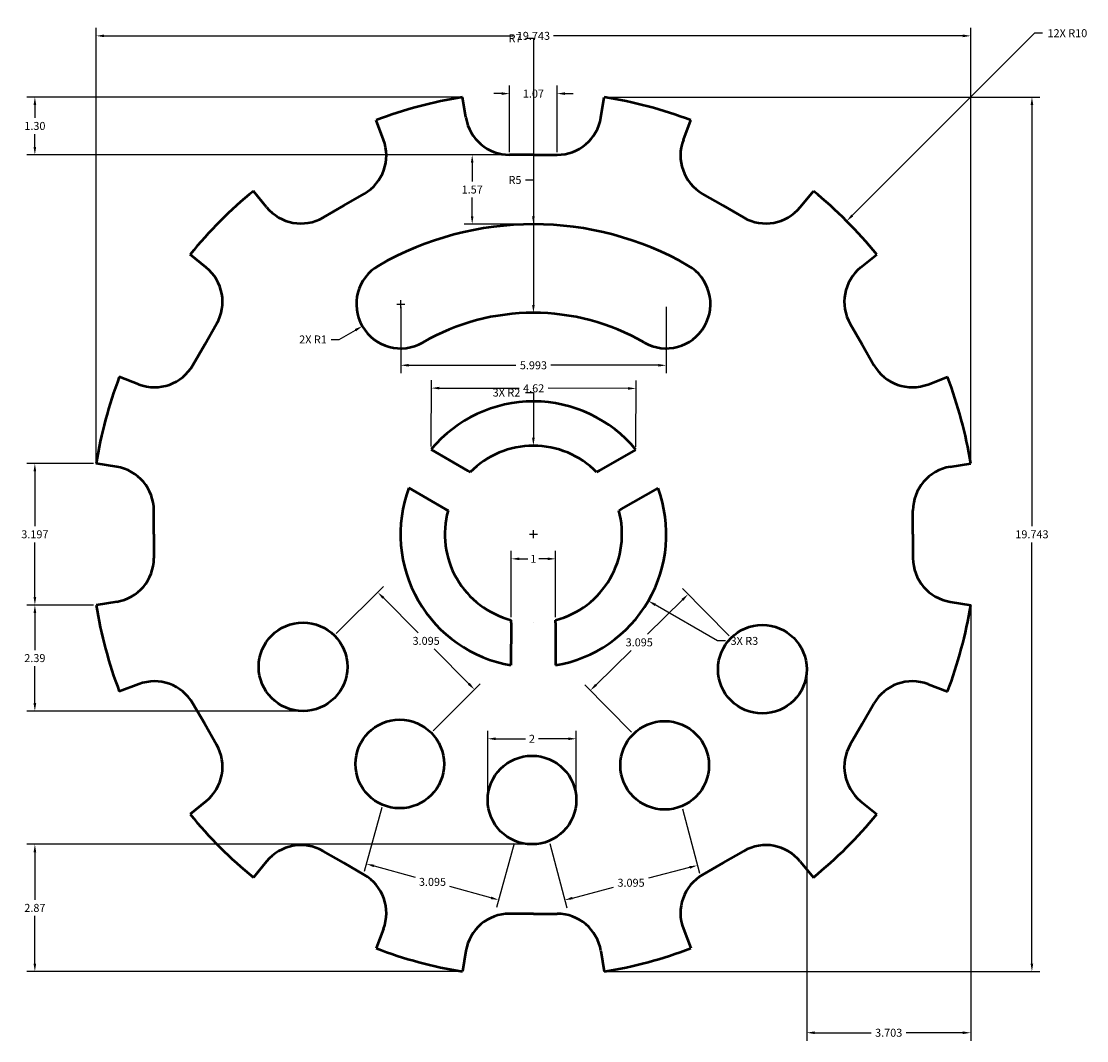
# Model space of a CAD drawing. Units: inches. Extents: x 14.9 to 39, y 2.3 to 25.3.
import ezdxf

# ---------------------------------------------------------------- set-up
doc = ezdxf.new("R2010")
doc.units = ezdxf.units.IN
doc.header["$MEASUREMENT"] = 0
for name, color, linetype, lineweight in [('M-CONS', 8, 'Continuous', 13), ('M-DIMS', 2, 'Continuous', 18), ('M-OUTL', 7, 'Continuous', 50)]:
    doc.layers.add(name, color=color, linetype=linetype, lineweight=lineweight)
doc.styles.get("Standard").update_dxf_attribs({"font": 'arial.ttf'})
doc.dimstyles.get("Standard").update_dxf_attribs({"dimtxt": 0.18, "dimasz": 0.18, "dimexe": 0.18, "dimexo": 0.0625, "dimgap": 0.09, "dimtad": 0, "dimtih": 1, "dimtoh": 1, "dimdec": 4, "dimzin": 0, "dimdsep": 46, "dimtxsty": 'Standard', "dimcen": 0.09, "dimadec": 0, "dimazin": 0, "dimtfac": 1, "dimtdec": 4, "dimtofl": 0, "dimtmove": 0, "dimatfit": 3, "dimfxl": 1, "dimtolj": 1, "dimtzin": 0, "dimarcsym": 0})

# ---------------------------------------------------------------- blocks, each defined once
blk = doc.blocks.new('*U1')
for p, q in [((-0.496, 0.479), (-0.504, -0.477)), ((0.504, 0.479), (0.501, -0.479))]:
    blk.add_line(p, q)
blk = doc.blocks.new('*U2')
at = {"layer": 'M-OUTL', "color": 0, "linetype": 'ByBlock', "lineweight": -2, "transparency": 16777216}
for p, rotation in [((24.356, 14.954), 240), ((28.65, 14.948), 120)]:
    blk.add_blockref('*U1', p, dxfattribs=dict(at, rotation=rotation))
blk.add_blockref('*U1', (26.498, 11.232), dxfattribs=at)
blk = doc.blocks.new('*U3')
blk.add_circle((0, 0), 1)
blk = doc.blocks.new('*U4')
at = {"layer": 'M-OUTL', "color": 0, "linetype": 'ByBlock', "lineweight": -2, "transparency": 16777216}
for p, rotation in [((31.67, 10.664), 119.5610080297864), ((23.484, 8.526), 29.89025200744661), ((29.464, 8.494), 89.67075602233986), ((26.469, 7.711), 59.78050401489326)]:
    blk.add_blockref('*U3', p, dxfattribs=dict(at, rotation=rotation))
blk.add_blockref('*U3', (21.301, 10.719), dxfattribs=at)
blk = doc.blocks.new('*U5')
for p, q in [((-1.523, 0.188), (-1.598, 0.652)), ((1.523, 0.188), (1.598, 0.652)), ((0, -0.652), (-0.536, -0.652)), ((0, -0.652), (0.536, -0.652))]:
    blk.add_line(p, q)
for centre, start, end in [((-0.536, 0.348), 189.1976, 270), ((0.536, 0.348), 270, 350.8024)]:
    blk.add_arc(centre, 1, start, end)
blk = doc.blocks.new('*U6')
at = {"layer": 'M-OUTL', "color": 0, "linetype": 'ByBlock', "lineweight": -2, "transparency": 16777216}
blk.add_blockref('*U5', (26.501, 22.931), dxfattribs=at)
for p, rotation in [((21.892, 21.696), 30), ((31.111, 21.696), 329.9999999999999), ((18.517, 18.321), 60), ((34.486, 18.321), 300), ((17.282, 13.711), 90), ((35.721, 13.711), 269.9999999999999), ((18.517, 9.102), 120), ((34.486, 9.102), 240), ((21.892, 5.727), 150), ((31.111, 5.727), 210), ((26.501, 4.492), 180)]:
    blk.add_blockref('*U5', p, dxfattribs=dict(at, rotation=rotation))
blk = doc.blocks.new('*D7')
at = {"layer": 'Defpoints', "color": 0, "transparency": 16777216}
for p in [(36.373, 24.965), (16.63, 15.31), (36.373, 15.31)]:
    blk.add_point(p, dxfattribs=at)
at = {"layer": 'M-DIMS', "color": 0, "lineweight": -2, "transparency": 16777216}
for p, q in [((16.63, 15.372), (16.63, 25.145)), ((36.373, 15.372), (36.373, 25.145)), ((16.81, 24.965), (26.046, 24.965)), ((36.193, 24.965), (26.957, 24.965))]:
    blk.add_line(p, q, dxfattribs=at)
at = {"layer": 'M-DIMS', "color": 0, "transparency": 16777216}
for points in [[(16.81, 24.995), (16.81, 24.935), (16.63, 24.965)], [(36.193, 24.995), (36.193, 24.935), (36.373, 24.965)]]:
    blk.add_solid(points, dxfattribs=at)
at = {"layer": 'M-DIMS', "color": 0, "transparency": 16777216, "insert": (26.501, 24.965), "char_height": 0.18, "attachment_point": 5}
blk.add_mtext('\\A1;19.743', dxfattribs=at)
blk = doc.blocks.new('*D8')
at = {"layer": 'Defpoints', "color": 0, "transparency": 16777216}
for p in [(28.1, 23.583), (37.755, 23.583), (28.1, 3.84)]:
    blk.add_point(p, dxfattribs=at)
at = {"layer": 'M-DIMS', "color": 0, "lineweight": -2, "transparency": 16777216}
for p, q in [((28.162, 23.583), (37.935, 23.583)), ((37.755, 23.403), (37.755, 13.893)), ((37.755, 4.02), (37.755, 13.529)), ((28.162, 3.84), (37.935, 3.84))]:
    blk.add_line(p, q, dxfattribs=at)
at = {"layer": 'M-DIMS', "color": 0, "transparency": 16777216}
for points in [[(37.725, 23.403), (37.785, 23.403), (37.755, 23.583)], [(37.725, 4.02), (37.785, 4.02), (37.755, 3.84)]]:
    blk.add_solid(points, dxfattribs=at)
at = {"layer": 'M-DIMS', "color": 0, "transparency": 16777216, "insert": (37.755, 13.711), "char_height": 0.18, "attachment_point": 5}
blk.add_mtext('\\A1;19.743', dxfattribs=at)
blk = doc.blocks.new('*D9')
at = {"layer": 'Defpoints', "color": 0, "transparency": 16777216}
for p in [(27.469, 9.094), (25.469, 7.711), (27.469, 7.711)]:
    blk.add_point(p, dxfattribs=at)
at = {"layer": 'M-DIMS', "color": 0, "lineweight": -2, "transparency": 16777216}
for p, q in [((25.469, 7.774), (25.469, 9.274)), ((27.469, 7.774), (27.469, 9.274)), ((25.649, 9.094), (26.32, 9.094)), ((27.289, 9.094), (26.619, 9.094))]:
    blk.add_line(p, q, dxfattribs=at)
at = {"layer": 'M-DIMS', "color": 0, "transparency": 16777216}
for points in [[(25.649, 9.124), (25.649, 9.064), (25.469, 9.094)], [(27.289, 9.124), (27.289, 9.064), (27.469, 9.094)]]:
    blk.add_solid(points, dxfattribs=at)
at = {"layer": 'M-DIMS', "color": 0, "transparency": 16777216, "insert": (26.469, 9.094), "char_height": 0.18, "attachment_point": 5}
blk.add_mtext('\\A1;2', dxfattribs=at)
blk = doc.blocks.new('*D10')
at = {"layer": 'Defpoints', "color": 0, "transparency": 16777216}
for p in [(23.505, 18.91), (29.498, 18.91), (23.505, 17.527)]:
    blk.add_point(p, dxfattribs=at)
at = {"layer": 'M-DIMS', "color": 0, "lineweight": -2, "transparency": 16777216}
for p, q in [((23.505, 18.847), (23.505, 17.347)), ((29.498, 18.847), (29.498, 17.347)), ((23.685, 17.527), (26.108, 17.527)), ((29.318, 17.527), (26.895, 17.527))]:
    blk.add_line(p, q, dxfattribs=at)
at = {"layer": 'M-DIMS', "color": 0, "transparency": 16777216}
for points in [[(23.685, 17.557), (23.685, 17.497), (23.505, 17.527)], [(29.318, 17.557), (29.318, 17.497), (29.498, 17.527)]]:
    blk.add_solid(points, dxfattribs=at)
at = {"layer": 'M-DIMS', "color": 0, "transparency": 16777216, "insert": (26.501, 17.527), "char_height": 0.18, "attachment_point": 5}
blk.add_mtext('\\A1;5.993', dxfattribs=at)
blk = doc.blocks.new('*D11')
at = {"layer": 'Defpoints', "color": 0, "transparency": 16777216}
for p in [(15.247, 15.31), (16.63, 15.31), (16.63, 12.113)]:
    blk.add_point(p, dxfattribs=at)
at = {"layer": 'M-DIMS', "color": 0, "lineweight": -2, "transparency": 16777216}
for p, q in [((16.567, 15.31), (15.067, 15.31)), ((15.247, 15.13), (15.247, 13.893)), ((15.247, 12.293), (15.247, 13.529)), ((16.567, 12.113), (15.067, 12.113))]:
    blk.add_line(p, q, dxfattribs=at)
at = {"layer": 'M-DIMS', "color": 0, "transparency": 16777216}
for points in [[(15.217, 15.13), (15.277, 15.13), (15.247, 15.31)], [(15.217, 12.293), (15.277, 12.293), (15.247, 12.113)]]:
    blk.add_solid(points, dxfattribs=at)
at = {"layer": 'M-DIMS', "color": 0, "transparency": 16777216, "insert": (15.247, 13.711), "char_height": 0.18, "attachment_point": 5}
blk.add_mtext('\\A1;3.197', dxfattribs=at)
blk = doc.blocks.new('*D12')
at = {"layer": 'Defpoints', "color": 0, "transparency": 16777216}
for p in [(24.903, 23.583), (15.247, 22.279), (25.965, 22.279)]:
    blk.add_point(p, dxfattribs=at)
at = {"layer": 'M-DIMS', "color": 0, "lineweight": -2, "transparency": 16777216}
for p, q in [((24.84, 23.583), (15.067, 23.583)), ((15.247, 23.403), (15.247, 23.113)), ((15.247, 22.459), (15.247, 22.749)), ((25.903, 22.279), (15.067, 22.279))]:
    blk.add_line(p, q, dxfattribs=at)
at = {"layer": 'M-DIMS', "color": 0, "transparency": 16777216}
for points in [[(15.217, 23.403), (15.277, 23.403), (15.247, 23.583)], [(15.217, 22.459), (15.277, 22.459), (15.247, 22.279)]]:
    blk.add_solid(points, dxfattribs=at)
at = {"layer": 'M-DIMS', "color": 0, "transparency": 16777216, "insert": (15.247, 22.931), "char_height": 0.18, "attachment_point": 5}
blk.add_mtext('\\A1;1.30', dxfattribs=at)
blk = doc.blocks.new('*D13')
at = {"layer": 'Defpoints', "color": 0, "transparency": 16777216}
for p in [(27.037, 23.661), (25.965, 22.279), (27.037, 22.279)]:
    blk.add_point(p, dxfattribs=at)
at = {"layer": 'M-DIMS', "color": 0, "lineweight": -2, "transparency": 16777216}
for p, q in [((25.965, 22.341), (25.965, 23.841)), ((27.037, 22.341), (27.037, 23.841)), ((25.785, 23.661), (25.605, 23.661)), ((27.217, 23.661), (27.397, 23.661))]:
    blk.add_line(p, q, dxfattribs=at)
at = {"layer": 'M-DIMS', "color": 0, "transparency": 16777216}
for points in [[(25.785, 23.691), (25.785, 23.631), (25.965, 23.661)], [(27.217, 23.691), (27.217, 23.631), (27.037, 23.661)]]:
    blk.add_solid(points, dxfattribs=at)
at = {"layer": 'M-DIMS', "color": 0, "transparency": 16777216, "insert": (26.501, 23.661), "char_height": 0.18, "attachment_point": 5}
blk.add_mtext('\\A1;1.07', dxfattribs=at)
blk = doc.blocks.new('*D14')
at = {"layer": 'Defpoints', "color": 0, "transparency": 16777216}
for p in [(27.001, 13.157), (26.001, 11.775), (27.001, 11.775)]:
    blk.add_point(p, dxfattribs=at)
at = {"layer": 'M-DIMS', "color": 0, "lineweight": -2, "transparency": 16777216}
for p, q in [((26.001, 11.837), (26.001, 13.337)), ((27.001, 11.837), (27.001, 13.337)), ((26.181, 13.157), (26.378, 13.157)), ((26.821, 13.157), (26.625, 13.157))]:
    blk.add_line(p, q, dxfattribs=at)
at = {"layer": 'M-DIMS', "color": 0, "transparency": 16777216}
for points in [[(26.181, 13.187), (26.181, 13.127), (26.001, 13.157)], [(26.821, 13.187), (26.821, 13.127), (27.001, 13.157)]]:
    blk.add_solid(points, dxfattribs=at)
at = {"layer": 'M-DIMS', "color": 0, "transparency": 16777216, "insert": (26.501, 13.157), "char_height": 0.18, "attachment_point": 5}
blk.add_mtext('\\A1;1', dxfattribs=at)
blk = doc.blocks.new('*D15')
at = {"layer": 'Defpoints', "color": 0, "transparency": 16777216}
for p in [(26.469, 6.711), (15.247, 3.84), (24.903, 3.84)]:
    blk.add_point(p, dxfattribs=at)
at = {"layer": 'M-DIMS', "color": 0, "lineweight": -2, "transparency": 16777216}
for p, q in [((26.407, 6.711), (15.067, 6.711)), ((15.247, 6.531), (15.247, 5.458)), ((15.247, 4.02), (15.247, 5.094)), ((24.84, 3.84), (15.067, 3.84))]:
    blk.add_line(p, q, dxfattribs=at)
at = {"layer": 'M-DIMS', "color": 0, "transparency": 16777216}
for points in [[(15.217, 6.531), (15.277, 6.531), (15.247, 6.711)], [(15.217, 4.02), (15.277, 4.02), (15.247, 3.84)]]:
    blk.add_solid(points, dxfattribs=at)
at = {"layer": 'M-DIMS', "color": 0, "transparency": 16777216, "insert": (15.247, 5.276), "char_height": 0.18, "attachment_point": 5}
blk.add_mtext('\\A1;2.87', dxfattribs=at)
blk = doc.blocks.new('*D16')
at = {"layer": 'Defpoints', "color": 0, "transparency": 16777216}
for p in [(22.008, 11.426), (25.171, 10.208), (24.191, 9.233)]:
    blk.add_point(p, dxfattribs=at)
at = {"layer": 'M-DIMS', "color": 0, "lineweight": -2, "transparency": 16777216}
for p, q in [((22.052, 11.471), (23.115, 12.529)), ((23.115, 12.274), (23.898, 11.487)), ((25.044, 10.335), (24.26, 11.123)), ((24.235, 9.277), (25.298, 10.335))]:
    blk.add_line(p, q, dxfattribs=at)
at = {"layer": 'M-DIMS', "color": 0, "transparency": 16777216}
for points in [[(23.136, 12.295), (23.093, 12.253), (22.988, 12.402)], [(25.065, 10.357), (25.022, 10.314), (25.171, 10.208)]]:
    blk.add_solid(points, dxfattribs=at)
at = {"layer": 'M-DIMS', "color": 0, "transparency": 16777216, "insert": (24.079, 11.305), "char_height": 0.18, "attachment_point": 5}
blk.add_mtext('\\A1;3.095', dxfattribs=at)
blk = doc.blocks.new('*D17')
at = {"layer": 'Defpoints', "color": 0, "transparency": 16777216}
for p in [(23.094, 7.604), (26.08, 6.79), (22.731, 6.27)]:
    blk.add_point(p, dxfattribs=at)
at = {"layer": 'M-DIMS', "color": 0, "lineweight": -2, "transparency": 16777216}
for p, q in [((23.078, 7.544), (22.683, 6.097)), ((26.064, 6.73), (25.669, 5.283)), ((22.904, 6.223), (23.829, 5.971)), ((25.543, 5.504), (24.618, 5.756))]:
    blk.add_line(p, q, dxfattribs=at)
at = {"layer": 'M-DIMS', "color": 0, "transparency": 16777216}
for points in [[(22.912, 6.252), (22.896, 6.194), (22.731, 6.27)], [(25.551, 5.533), (25.535, 5.475), (25.716, 5.456)]]:
    blk.add_solid(points, dxfattribs=at)
at = {"layer": 'M-DIMS', "color": 0, "transparency": 16777216, "insert": (24.223, 5.863), "char_height": 0.18, "attachment_point": 5}
blk.add_mtext('\\A1;3.095', dxfattribs=at)
blk = doc.blocks.new('*D18')
at = {"layer": 'Defpoints', "color": 0, "transparency": 16777216}
for p in [(29.853, 7.572), (26.859, 6.79), (27.208, 5.452)]:
    blk.add_point(p, dxfattribs=at)
at = {"layer": 'M-DIMS', "color": 0, "lineweight": -2, "transparency": 16777216}
for p, q in [((29.869, 7.512), (30.248, 6.06)), ((26.874, 6.73), (27.253, 5.278)), ((30.028, 6.189), (29.099, 5.946)), ((27.382, 5.498), (28.311, 5.741))]:
    blk.add_line(p, q, dxfattribs=at)
at = {"layer": 'M-DIMS', "color": 0, "transparency": 16777216}
for points in [[(30.02, 6.218), (30.036, 6.16), (30.202, 6.235)], [(27.374, 5.527), (27.39, 5.469), (27.208, 5.452)]]:
    blk.add_solid(points, dxfattribs=at)
at = {"layer": 'M-DIMS', "color": 0, "transparency": 16777216, "insert": (28.705, 5.843), "char_height": 0.18, "attachment_point": 5}
blk.add_mtext('\\A1;3.095', dxfattribs=at)
blk = doc.blocks.new('*D19')
at = {"layer": 'Defpoints', "color": 0, "transparency": 16777216}
for p in [(29.993, 12.357), (30.963, 11.371), (28.756, 9.201)]:
    blk.add_point(p, dxfattribs=at)
at = {"layer": 'M-DIMS', "color": 0, "lineweight": -2, "transparency": 16777216}
for p, q in [((30.919, 11.415), (29.867, 12.485)), ((29.865, 12.23), (29.075, 11.453)), ((27.915, 10.313), (28.705, 11.089)), ((28.713, 9.245), (27.661, 10.315))]:
    blk.add_line(p, q, dxfattribs=at)
at = {"layer": 'M-DIMS', "color": 0, "transparency": 16777216}
for points in [[(29.844, 12.252), (29.886, 12.209), (29.993, 12.357)], [(27.894, 10.334), (27.936, 10.291), (27.787, 10.186)]]:
    blk.add_solid(points, dxfattribs=at)
at = {"layer": 'M-DIMS', "color": 0, "transparency": 16777216, "insert": (28.89, 11.271), "char_height": 0.18, "attachment_point": 5}
blk.add_mtext('\\A1;3.095', dxfattribs=at)
blk = doc.blocks.new('*D20')
at = {"layer": 'Defpoints', "color": 0, "transparency": 16777216}
for p in [(36.373, 12.113), (32.67, 10.664), (36.373, 2.457)]:
    blk.add_point(p, dxfattribs=at)
at = {"layer": 'M-DIMS', "color": 0, "lineweight": -2, "transparency": 16777216}
for p, q in [((36.373, 12.051), (36.373, 2.277)), ((32.67, 10.601), (32.67, 2.277)), ((32.85, 2.457), (34.128, 2.457)), ((36.193, 2.457), (34.915, 2.457))]:
    blk.add_line(p, q, dxfattribs=at)
at = {"layer": 'M-DIMS', "color": 0, "transparency": 16777216}
for points in [[(32.85, 2.487), (32.85, 2.427), (32.67, 2.457)], [(36.193, 2.487), (36.193, 2.427), (36.373, 2.457)]]:
    blk.add_solid(points, dxfattribs=at)
at = {"layer": 'M-DIMS', "color": 0, "transparency": 16777216, "insert": (34.521, 2.457), "char_height": 0.18, "attachment_point": 5}
blk.add_mtext('\\A1;3.703', dxfattribs=at)
blk = doc.blocks.new('*D21')
at = {"layer": 'Defpoints', "color": 0, "transparency": 16777216}
for p in [(16.63, 12.113), (15.247, 9.719), (21.301, 9.719)]:
    blk.add_point(p, dxfattribs=at)
at = {"layer": 'M-DIMS', "color": 0, "lineweight": -2, "transparency": 16777216}
for p, q in [((16.567, 12.113), (15.067, 12.113)), ((15.247, 11.933), (15.247, 11.098)), ((15.247, 9.899), (15.247, 10.734)), ((21.238, 9.719), (15.067, 9.719))]:
    blk.add_line(p, q, dxfattribs=at)
at = {"layer": 'M-DIMS', "color": 0, "transparency": 16777216}
for points in [[(15.217, 11.933), (15.277, 11.933), (15.247, 12.113)], [(15.217, 9.899), (15.277, 9.899), (15.247, 9.719)]]:
    blk.add_solid(points, dxfattribs=at)
at = {"layer": 'M-DIMS', "color": 0, "transparency": 16777216, "insert": (15.247, 10.916), "char_height": 0.18, "attachment_point": 5}
blk.add_mtext('\\A1;2.39', dxfattribs=at)
blk = doc.blocks.new('*D22')
at = {"layer": 'Defpoints', "color": 0, "transparency": 16777216}
for p in [(25.119, 22.279), (26.501, 22.279), (26.501, 20.711)]:
    blk.add_point(p, dxfattribs=at)
at = {"layer": 'M-DIMS', "color": 0, "lineweight": -2, "transparency": 16777216}
for p, q in [((26.439, 22.279), (24.939, 22.279)), ((25.119, 22.099), (25.119, 21.677)), ((25.119, 20.891), (25.119, 21.313)), ((26.439, 20.711), (24.939, 20.711))]:
    blk.add_line(p, q, dxfattribs=at)
at = {"layer": 'M-DIMS', "color": 0, "transparency": 16777216}
for points in [[(25.089, 22.099), (25.149, 22.099), (25.119, 22.279)], [(25.089, 20.891), (25.149, 20.891), (25.119, 20.711)]]:
    blk.add_solid(points, dxfattribs=at)
at = {"layer": 'M-DIMS', "color": 0, "transparency": 16777216, "insert": (25.119, 21.495), "char_height": 0.18, "attachment_point": 5}
blk.add_mtext('\\A1;1.57', dxfattribs=at)
blk = doc.blocks.new('*D23')
at = {"layer": 'Defpoints', "color": 0, "transparency": 16777216}
for p in [(28.817, 17.004), (24.195, 15.629), (28.815, 15.621)]:
    blk.add_point(p, dxfattribs=at)
at = {"layer": 'M-DIMS', "color": 0, "lineweight": -2, "transparency": 16777216}
for p, q in [((24.195, 15.692), (24.197, 17.192)), ((28.815, 15.684), (28.818, 17.184)), ((24.377, 17.012), (26.181, 17.008)), ((28.637, 17.004), (26.834, 17.007))]:
    blk.add_line(p, q, dxfattribs=at)
at = {"layer": 'M-DIMS', "color": 0, "transparency": 16777216}
for points in [[(24.377, 17.042), (24.377, 16.982), (24.197, 17.012)], [(28.637, 17.034), (28.637, 16.974), (28.817, 17.004)]]:
    blk.add_solid(points, dxfattribs=at)
at = {"layer": 'M-DIMS', "color": 0, "transparency": 16777216, "insert": (26.507, 17.008), "char_height": 0.18, "attachment_point": 5}
blk.add_mtext('\\A1;4.62', dxfattribs=at)
blk = doc.blocks.new('*D24')
at = {"layer": 'Defpoints', "color": 0, "transparency": 16777216}
for p in [(33.572, 20.782), (26.501, 13.711)]:
    blk.add_point(p, dxfattribs=at)
at = {"layer": 'M-DIMS', "color": 0, "lineweight": -2, "transparency": 16777216}
for p, q in [((37.815, 25.025), (33.7, 20.91)), ((37.995, 25.025), (37.815, 25.025)), ((26.411, 13.711), (26.591, 13.711)), ((26.501, 13.621), (26.501, 13.801))]:
    blk.add_line(p, q, dxfattribs=at)
at = {"layer": 'M-DIMS', "color": 0, "transparency": 16777216}
blk.add_solid([(33.679, 20.931), (33.721, 20.889), (33.572, 20.782)], dxfattribs=at)
at = {"layer": 'M-DIMS', "color": 0, "transparency": 16777216, "insert": (38.555, 25.025), "char_height": 0.18, "attachment_point": 5}
blk.add_mtext('\\A1;12X R10', dxfattribs=at)
blk = doc.blocks.new('*D25')
at = {"layer": 'Defpoints', "color": 0, "transparency": 16777216}
for p in [(26.501, 20.711), (26.501, 13.711)]:
    blk.add_point(p, dxfattribs=at)
at = {"layer": 'M-DIMS', "color": 0, "lineweight": -2, "transparency": 16777216}
for p, q in [((26.321, 24.911), (26.501, 24.911)), ((26.501, 24.911), (26.501, 20.891)), ((26.411, 13.711), (26.591, 13.711)), ((26.501, 13.621), (26.501, 13.801))]:
    blk.add_line(p, q, dxfattribs=at)
at = {"layer": 'M-DIMS', "color": 0, "transparency": 16777216}
blk.add_solid([(26.531, 20.891), (26.471, 20.891), (26.501, 20.711)], dxfattribs=at)
at = {"layer": 'M-DIMS', "color": 0, "transparency": 16777216, "insert": (26.086, 24.911), "char_height": 0.18, "attachment_point": 5}
blk.add_mtext('\\A1;R7', dxfattribs=at)
blk = doc.blocks.new('*D26')
at = {"layer": 'Defpoints', "color": 0, "transparency": 16777216}
for p in [(26.501, 18.711), (26.501, 13.711)]:
    blk.add_point(p, dxfattribs=at)
at = {"layer": 'M-DIMS', "color": 0, "lineweight": -2, "transparency": 16777216}
for p, q in [((26.321, 21.711), (26.501, 21.711)), ((26.501, 21.711), (26.501, 18.891)), ((26.411, 13.711), (26.591, 13.711)), ((26.501, 13.621), (26.501, 13.801))]:
    blk.add_line(p, q, dxfattribs=at)
at = {"layer": 'M-DIMS', "color": 0, "transparency": 16777216}
blk.add_solid([(26.531, 18.891), (26.471, 18.891), (26.501, 18.711)], dxfattribs=at)
at = {"layer": 'M-DIMS', "color": 0, "transparency": 16777216, "insert": (26.085, 21.711), "char_height": 0.18, "attachment_point": 5}
blk.add_mtext('\\A1;R5', dxfattribs=at)
blk = doc.blocks.new('*D27')
at = {"layer": 'Defpoints', "color": 0, "transparency": 16777216}
for p in [(23.505, 18.91), (22.639, 18.41)]:
    blk.add_point(p, dxfattribs=at)
at = {"layer": 'M-DIMS', "color": 0, "lineweight": -2, "transparency": 16777216}
for p, q in [((23.415, 18.91), (23.595, 18.91)), ((23.505, 18.82), (23.505, 19)), ((22.119, 18.11), (22.483, 18.32)), ((21.939, 18.11), (22.119, 18.11))]:
    blk.add_line(p, q, dxfattribs=at)
at = {"layer": 'M-DIMS', "color": 0, "transparency": 16777216}
blk.add_solid([(22.468, 18.346), (22.498, 18.294), (22.639, 18.41)], dxfattribs=at)
at = {"layer": 'M-DIMS', "color": 0, "transparency": 16777216, "insert": (21.526, 18.11), "char_height": 0.18, "attachment_point": 5}
blk.add_mtext('\\A1;2X R1', dxfattribs=at)
blk = doc.blocks.new('*D28')
at = {"layer": 'Defpoints', "color": 0, "transparency": 16777216}
for p in [(26.501, 13.711), (29.097, 12.207)]:
    blk.add_point(p, dxfattribs=at)
at = {"layer": 'M-DIMS', "color": 0, "lineweight": -2, "transparency": 16777216}
for p, q in [((26.411, 13.711), (26.591, 13.711)), ((26.501, 13.621), (26.501, 13.801)), ((30.654, 11.304), (29.253, 12.117)), ((30.834, 11.304), (30.654, 11.304))]:
    blk.add_line(p, q, dxfattribs=at)
at = {"layer": 'M-DIMS', "color": 0, "transparency": 16777216}
blk.add_solid([(29.268, 12.143), (29.238, 12.091), (29.097, 12.207)], dxfattribs=at)
at = {"layer": 'M-DIMS', "color": 0, "transparency": 16777216, "insert": (31.263, 11.304), "char_height": 0.18, "attachment_point": 5}
blk.add_mtext('\\A1;3X R3', dxfattribs=at)
blk = doc.blocks.new('*D29')
at = {"layer": 'Defpoints', "color": 0, "transparency": 16777216}
for p in [(26.501, 15.711), (26.501, 13.711)]:
    blk.add_point(p, dxfattribs=at)
at = {"layer": 'M-DIMS', "color": 0, "lineweight": -2, "transparency": 16777216}
for p, q in [((26.321, 16.911), (26.501, 16.911)), ((26.501, 16.911), (26.501, 15.891)), ((26.411, 13.711), (26.591, 13.711)), ((26.501, 13.621), (26.501, 13.801))]:
    blk.add_line(p, q, dxfattribs=at)
at = {"layer": 'M-DIMS', "color": 0, "transparency": 16777216}
blk.add_solid([(26.531, 15.891), (26.471, 15.891), (26.501, 15.711)], dxfattribs=at)
at = {"layer": 'M-DIMS', "color": 0, "transparency": 16777216, "insert": (25.893, 16.911), "char_height": 0.18, "attachment_point": 5}
blk.add_mtext('\\A1;3X R2', dxfattribs=at)

msp = doc.modelspace()

# ---------------------------------------------------------------- linework, layer by layer
at = {"layer": 'M-CONS'}
for p, q in [((26.5014, 22.2786), (26.5014, 22.2786)), ((26.5014, 11.7114), (26.5014, 11.7114))]:
    msp.add_line(p, q, dxfattribs=at)
at = {"layer": 'M-OUTL'}
for p, q in [((25.0193, 15.1444), (25.074, 15.1123)), ((27.9834, 15.1444), (27.9283, 15.1128)), ((24.5193, 14.2784), (24.5743, 14.2465)), ((28.4834, 14.2784), (28.4286, 14.2462)), ((26.0014, 11.7114), (26.0014, 11.7749)), ((27.0014, 11.7114), (27.0014, 11.7749))]:
    msp.add_line(p, q, dxfattribs=at)
for centre, radius, start, end in [((26.5014, 13.7114), 10, 99.1976, 110.8024), ((26.5014, 13.7114), 10, 69.1976, 80.8024), ((26.5014, 13.7114), 10, 129.1976, 140.8024), ((26.5014, 13.7114), 10, 39.1976, 50.8024), ((26.5014, 13.7114), 7, 60.03846, 119.96154), ((23.5049, 18.9096), 1, 119.96154, 299.96154), ((29.4979, 18.9096), 1, 240.03846, 60.03846), ((26.5014, 13.7114), 5, 60.03846, 119.96154), ((26.5014, 13.7114), 10, 159.1976, 170.8024), ((26.5014, 13.7114), 10, 9.1976, 20.8024), ((26.5014, 13.7114), 3, 39.54266, 140.25795), ((26.5014, 13.7114), 2, 44.48272, 135.53746), ((26.5014, 13.7114), 3, 159.54266, 260.25795), ((26.5014, 13.7114), 3, 279.54266, 20.25795), ((26.5014, 13.7114), 2, 164.48272, 255.52249), ((26.5014, 13.7114), 2, 284.47751, 15.5098), ((26.5014, 13.7114), 10, 189.1976, 200.8024), ((26.5014, 13.7114), 10, 339.1976, 350.8024), ((26.5014, 13.7114), 10, 219.1976, 230.8024), ((26.5014, 13.7114), 10, 309.1976, 320.8024), ((26.5014, 13.7114), 10, 249.1976, 260.8024), ((26.5014, 13.7114), 10, 279.1976, 290.8024)]:
    msp.add_arc(centre, radius, start, end, dxfattribs=at)

# ---------------------------------------------------------------- block references
for name in ['*U6', '*U2', '*U4']:
    msp.add_blockref(name, (0, 0), dxfattribs=at)

# ---------------------------------------------------------------- dimensions: what is measured, and where the dimension line sits
at = {"layer": 'M-DIMS'}
for center, mpoint, text, picture, middle in [((26.5014, 13.7114), (33.5725, 20.7825), '12X <>', '*D24', (38.5547, 25.0251)), ((23.5049, 18.9096), (22.6387, 18.4098), '2X <>', '*D27', (21.5263, 18.11)), ((26.5014, 13.7114), (26.501, 15.7114), '3X <>', '*D29', (25.8932, 16.9114)), ((26.5014, 13.7114), (29.0969, 12.207), '3X <>', '*D28', (31.2627, 11.3044))]:
    dim = msp.add_radius_dim(center=center, mpoint=mpoint, text=text, dimstyle='Standard', override={"dimdec": 0, "dimlfac": 1, "dimrnd": 0, "dimzin": 0, "dimdsep": 46, "dimlunit": 2}, dxfattribs=at)
    dim.commit()
    dim.dimension.update_dxf_attribs({"geometry": picture, "text_midpoint": middle, "dimtype": 164})
for base, p1, p2, override, picture, middle in [((36.3728, 24.9653), (16.63, 15.3098), (36.3728, 15.3098), {"dimdec": 3, "dimlfac": 1, "dimrnd": 0, "dimzin": 0, "dimdsep": 46, "dimlunit": 2}, '*D7', (26.5014, 24.9653)), ((36.3728, 2.4575), (32.6698, 10.6638), (36.3728, 12.113), {"dimdec": 3, "dimlfac": 1, "dimrnd": 0, "dimzin": 0, "dimdsep": 46, "dimlunit": 2}, '*D20', (34.5213, 2.4575)), ((27.4693, 9.094), (25.4693, 7.7115), (27.4693, 7.7115), {"dimdec": 0, "dimlfac": 1, "dimrnd": 0, "dimzin": 0, "dimdsep": 46, "dimlunit": 2}, '*D9', (26.4693, 9.094))]:
    dim = msp.add_linear_dim(base=base, p1=p1, p2=p2, dimstyle='Standard', override=override, dxfattribs=at)
    dim.commit()
    dim.dimension.update_dxf_attribs({"geometry": picture, "text_midpoint": middle})
for mpoint, picture, middle in [((26.501, 20.7114), '*D25', (26.0856, 24.9114)), ((26.501, 18.7114), '*D26', (26.085, 21.7114))]:
    dim = msp.add_radius_dim(center=(26.5014, 13.7114), mpoint=mpoint, dimstyle='Standard', override={"dimdec": 0, "dimlfac": 1, "dimrnd": 0, "dimzin": 0, "dimdsep": 46, "dimlunit": 2}, dxfattribs=at)
    dim.commit()
    dim.dimension.update_dxf_attribs({"geometry": picture, "text_midpoint": middle, "dimtype": 164})
for base, p1, p2, angle, override, picture, middle in [((27.0375, 23.6611), (25.9653, 22.2786), (27.0375, 22.2786), 0, {"dimdec": 2, "dimlfac": 1, "dimrnd": 0, "dimzin": 0, "dimdsep": 46, "dimlunit": 2}, '*D13', (26.5014, 23.6611)), ((15.2475, 22.2786), (24.903, 23.5828), (25.9653, 22.2786), 90, {"dimdec": 2, "dimlfac": 1, "dimrnd": 0, "dimzin": 0, "dimdsep": 46, "dimlunit": 2}, '*D12', (15.2475, 22.9307)), ((37.7553, 23.5828), (28.0998, 3.84), (28.0998, 23.5828), 90, {"dimdec": 3, "dimlfac": 1, "dimrnd": 0, "dimzin": 0, "dimdsep": 46, "dimlunit": 2}, '*D8', (37.7553, 13.7114)), ((25.1189, 22.2786), (26.5014, 20.7114), (26.5014, 22.2786), 90, {"dimdec": 2, "dimlfac": 1, "dimrnd": 0, "dimzin": 0, "dimdsep": 46, "dimlunit": 2}, '*D22', (25.1189, 21.495)), ((23.5049, 17.5271), (29.4979, 18.9096), (23.5049, 18.9096), 180, {"dimdec": 3, "dimlfac": 1, "dimrnd": 0, "dimzin": 0, "dimdsep": 46, "dimlunit": 2}, '*D10', (26.5014, 17.5271)), ((28.8172, 17.0039), (24.1946, 15.6294), (28.8148, 15.6214), 359.90031, {"dimdec": 2, "dimlfac": 1, "dimrnd": 0, "dimzin": 0, "dimdsep": 46, "dimlunit": 2}, '*D23', (26.5071, 17.0079)), ((15.2475, 15.3098), (16.63, 12.113), (16.63, 15.3098), 90, {"dimdec": 3, "dimlfac": 1, "dimrnd": 0, "dimzin": 0, "dimdsep": 46, "dimlunit": 2}, '*D11', (15.2475, 13.7114)), ((27.0014, 13.1574), (26.0014, 11.7749), (27.0014, 11.7749), 0, {"dimdec": 0, "dimlfac": 1, "dimrnd": 0, "dimzin": 0, "dimdsep": 46, "dimlunit": 2}, '*D14', (26.5014, 13.1574)), ((25.1706, 10.2078), (22.0078, 11.4264), (24.1907, 9.2327), 314.85794, {"dimdec": 3, "dimlfac": 1, "dimrnd": 0, "dimzin": 0, "dimdsep": 46, "dimlunit": 2}, '*D16', (24.0792, 11.3047)), ((29.9932, 12.3565), (28.7564, 9.2007), (30.9627, 11.3709), 44.52869, {"dimdec": 3, "dimlfac": 1, "dimrnd": 0, "dimzin": 0, "dimdsep": 46, "dimlunit": 2}, '*D19', (28.89, 11.2714)), ((15.2475, 9.7193), (16.63, 12.113), (21.3007, 9.7193), 90, {"dimdec": 2, "dimlfac": 1, "dimrnd": 0, "dimzin": 0, "dimdsep": 46, "dimlunit": 2}, '*D21', (15.2475, 10.9162)), ((22.7306, 6.2704), (26.08, 6.7901), (23.0943, 7.6042), 164.74819, {"dimdec": 3, "dimlfac": 1, "dimrnd": 0, "dimzin": 0, "dimdsep": 46, "dimlunit": 2}, '*D17', (24.2235, 5.8633)), ((27.2079, 5.4524), (29.8528, 7.5722), (26.8585, 6.7901), 194.63844, {"dimdec": 3, "dimlfac": 1, "dimrnd": 0, "dimzin": 0, "dimdsep": 46, "dimlunit": 2}, '*D18', (28.705, 5.8435)), ((15.2475, 3.84), (26.4693, 6.7115), (24.903, 3.84), 90, {"dimdec": 2, "dimlfac": 1, "dimrnd": 0, "dimzin": 0, "dimdsep": 46, "dimlunit": 2}, '*D15', (15.2475, 5.2757))]:
    dim = msp.add_linear_dim(base=base, p1=p1, p2=p2, angle=angle, dimstyle='Standard', override=override, dxfattribs=at)
    dim.commit()
    dim.dimension.update_dxf_attribs({"geometry": picture, "text_midpoint": middle})

doc.saveas('drawing.dxf')
